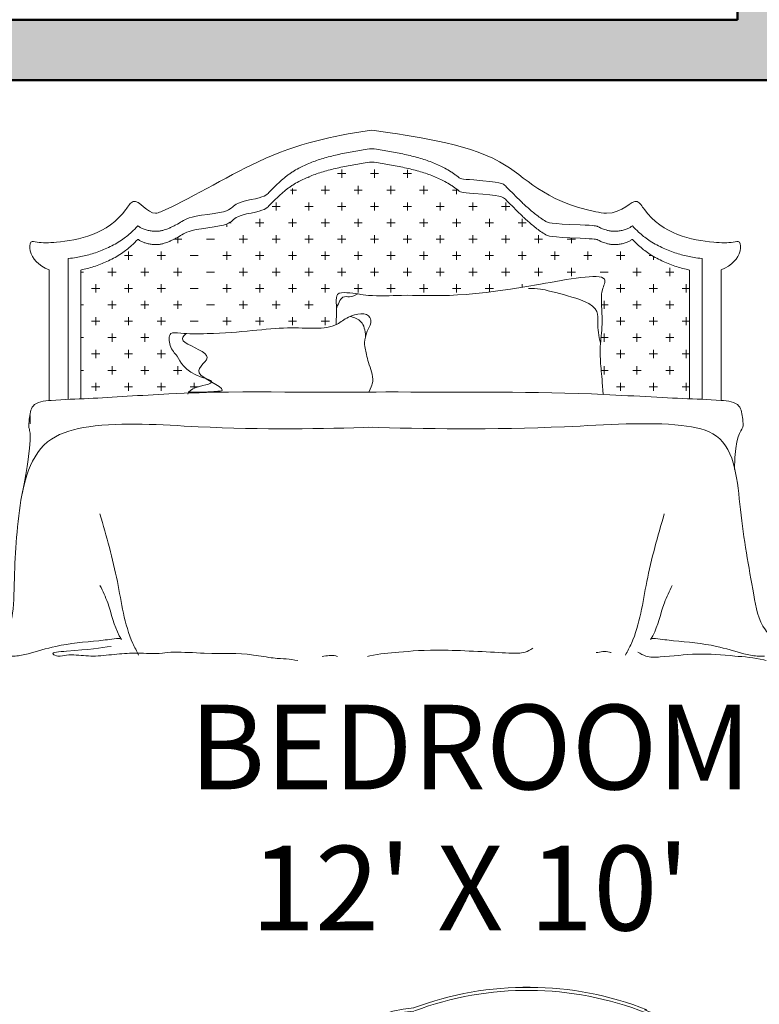
# Model space of a CAD drawing. Units: inches. Extents: x 1771 to 3025, y 319 to 889.
# Tile 10 of 35: x 1978 to 2040, y 713 to 795. Entities that reach past the tile are written whole.
import ezdxf

# ---------------------------------------------------------------- set-up
doc = ezdxf.new("R2010")
doc.units = ezdxf.units.IN
doc.header["$MEASUREMENT"] = 0
doc.set_wipeout_variables(frame=1)
for name, color, linetype, lineweight in [('A-AREA-IDEN', 241, 'Continuous', 25), ('A-FURN', 8, 'Continuous', 18), ('A-WALL', 7, 'Continuous', 50), ('A-WALL-PATT', 254, 'Continuous', 13)]:
    doc.layers.add(name, color=color, linetype=linetype, lineweight=lineweight)
doc.styles.get("Standard").update_dxf_attribs({"font": 'arial.ttf'})

# ---------------------------------------------------------------- blocks, each defined once
blk = doc.blocks.new('A$C3F6F0378')
for p, q in [((1262.2, 944.7), (1262.2, 960.5)), ((1325.7, 944.7), (1325.7, 960.5)), ((1389.2, 944.7), (1389.2, 959.9)), ((1198.7, 944.7), (1198.7, 946.2)), ((1254.2, 952.6), (1270.1, 952.6)), ((1317.7, 952.6), (1333.6, 952.6)), ((1381.2, 952.6), (1397.1, 952.6)), ((1162.7, 920.9), (1174.9, 920.9)), ((1166.9, 912.9), (1166.9, 924)), ((1222.5, 920.9), (1238.4, 920.9)), ((1230.4, 912.9), (1230.4, 928.8)), ((1286, 920.9), (1301.9, 920.9)), ((1293.9, 912.9), (1293.9, 928.8)), ((1349.5, 920.9), (1365.4, 920.9)), ((1357.4, 912.9), (1357.4, 928.8)), ((1413, 920.9), (1428.9, 920.9)), ((1420.9, 912.9), (1420.9, 928.8)), ((1476.5, 920.9), (1485.8, 920.9)), ((1484.4, 912.9), (1484.4, 921.6)), ((1135.2, 881.2), (1135.2, 897)), ((1198.7, 881.2), (1198.7, 897)), ((1262.2, 881.2), (1262.2, 897)), ((1325.7, 881.2), (1325.7, 897)), ((1389.2, 881.2), (1389.2, 897)), ((1452.7, 881.2), (1452.7, 897)), ((1516.2, 881.2), (1516.2, 897)), ((1579.7, 881.2), (1579.7, 897)), ((1127.2, 889.1), (1143.1, 889.1)), ((1190.7, 889.1), (1206.6, 889.1)), ((1254.2, 889.1), (1270.1, 889.1)), ((1317.7, 889.1), (1333.6, 889.1)), ((1381.2, 889.1), (1397.1, 889.1)), ((1444.7, 889.1), (1460.6, 889.1)), ((1508.2, 889.1), (1524.1, 889.1)), ((1571.7, 889.1), (1587.6, 889.1)), ((1103.4, 849.4), (1103.4, 865.3)), ((1166.9, 849.4), (1166.9, 865.3)), ((1230.4, 849.4), (1230.4, 865.3)), ((1293.9, 849.4), (1293.9, 865.3)), ((1357.4, 849.4), (1357.4, 865.3)), ((1420.9, 849.4), (1420.9, 865.3)), ((1484.4, 849.4), (1484.4, 865.3)), ((1547.9, 849.4), (1547.9, 865.3)), ((1611.4, 849.4), (1611.4, 865.3)), ((1039.9, 849.4), (1039.9, 855.2)), ((1044.6, 857.4), (1047.9, 857.4)), ((1095.5, 857.4), (1111.4, 857.4)), ((1159, 857.4), (1174.9, 857.4)), ((1222.5, 857.4), (1238.4, 857.4)), ((1286, 857.4), (1301.9, 857.4)), ((1349.5, 857.4), (1365.4, 857.4)), ((1413, 857.4), (1428.9, 857.4)), ((1476.5, 857.4), (1492.4, 857.4)), ((1540, 857.4), (1555.9, 857.4)), ((1603.5, 857.4), (1619.4, 857.4)), ((937.5, 825.6), (952.6, 825.6)), ((944.7, 817.7), (944.7, 829.4)), ((1000.2, 825.6), (1016.1, 825.6)), ((1063.7, 825.6), (1079.6, 825.6)), ((1071.7, 817.7), (1071.7, 833.5)), ((1127.2, 825.6), (1143.1, 825.6)), ((1135.2, 817.7), (1135.2, 833.5)), ((1190.7, 825.6), (1206.6, 825.6)), ((1198.7, 817.7), (1198.7, 833.5)), ((1254.2, 825.6), (1270.1, 825.6)), ((1262.2, 817.7), (1262.2, 833.5)), ((1317.7, 825.6), (1333.6, 825.6)), ((1325.7, 817.7), (1325.7, 833.5)), ((1381.2, 825.6), (1397.1, 825.6)), ((1389.2, 817.7), (1389.2, 833.5)), ((1444.7, 825.6), (1460.6, 825.6)), ((1452.7, 817.7), (1452.7, 833.5)), ((1508.2, 825.6), (1524.1, 825.6)), ((1516.2, 817.7), (1516.2, 833.5)), ((1571.7, 825.6), (1587.6, 825.6)), ((1579.7, 817.7), (1579.7, 833.5)), ((1635.2, 825.6), (1651.1, 825.6)), ((1643.2, 817.7), (1643.2, 833.5)), ((1698.7, 825.6), (1714.6, 825.6)), ((1706.7, 817.7), (1706.7, 828.2)), ((849.4, 785.9), (849.4, 801.8)), ((881.2, 817.7), (881.2, 818.8)), ((912.9, 785.9), (912.9, 801.8)), ((1039.9, 785.9), (1039.9, 801.8)), ((1103.4, 785.9), (1103.4, 801.8)), ((1166.9, 785.9), (1166.9, 801.8)), ((1230.4, 785.9), (1230.4, 801.8)), ((1293.9, 785.9), (1293.9, 801.8)), ((1357.4, 785.9), (1357.4, 801.8)), ((1420.9, 785.9), (1420.9, 801.8)), ((1484.4, 785.9), (1484.4, 801.8)), ((1547.9, 785.9), (1547.9, 801.8)), ((1611.4, 785.9), (1611.4, 801.8)), ((1674.9, 785.9), (1674.9, 801.8)), ((1738.4, 785.9), (1738.4, 801.8)), ((1770.2, 818.9), (1770.2, 818.9)), ((1801.9, 785.9), (1801.9, 801.8)), ((841.5, 793.9), (857.4, 793.9)), ((905, 793.9), (920.9, 793.9)), ((968.5, 793.9), (984.4, 793.9)), ((1032, 793.9), (1047.9, 793.9)), ((1095.5, 793.9), (1111.4, 793.9)), ((1159, 793.9), (1174.9, 793.9)), ((1222.5, 793.9), (1238.4, 793.9)), ((1286, 793.9), (1301.9, 793.9)), ((1349.5, 793.9), (1365.4, 793.9)), ((1413, 793.9), (1428.9, 793.9)), ((1476.5, 793.9), (1492.4, 793.9)), ((1540, 793.9), (1555.9, 793.9)), ((1603.5, 793.9), (1619.4, 793.9)), ((1667, 793.9), (1682.9, 793.9)), ((1730.5, 793.9), (1746.4, 793.9)), ((1794, 793.9), (1809.9, 793.9)), ((1857.5, 793.9), (1863, 793.9)), ((1865.4, 785.9), (1865.4, 792.4)), ((817.7, 754.2), (817.7, 770)), ((881.2, 754.2), (881.2, 770)), ((944.7, 754.2), (944.7, 770)), ((1071.7, 754.2), (1071.7, 770)), ((1135.2, 754.2), (1135.2, 770)), ((1198.7, 754.2), (1198.7, 770)), ((1262.2, 754.2), (1262.2, 770)), ((1325.7, 754.2), (1325.7, 770)), ((1389.2, 754.2), (1389.2, 770)), ((1452.7, 754.2), (1452.7, 770)), ((1516.2, 754.2), (1516.2, 770)), ((1579.7, 754.2), (1579.7, 770)), ((1643.2, 754.2), (1643.2, 770)), ((1706.7, 754.2), (1706.7, 770)), ((1833.7, 754.2), (1833.7, 770)), ((1897.2, 754.2), (1897.2, 770)), ((757.1, 762.1), (762.1, 762.1)), ((809.7, 762.1), (825.6, 762.1)), ((873.2, 762.1), (889.1, 762.1)), ((936.7, 762.1), (952.6, 762.1)), ((1000.2, 762.1), (1016.1, 762.1)), ((1063.7, 762.1), (1079.6, 762.1)), ((1127.2, 762.1), (1143.1, 762.1)), ((1190.7, 762.1), (1206.6, 762.1)), ((1254.2, 762.1), (1270.1, 762.1)), ((1317.7, 762.1), (1333.6, 762.1)), ((1381.2, 762.1), (1397.1, 762.1)), ((1444.7, 762.1), (1460.6, 762.1)), ((1508.2, 762.1), (1524.1, 762.1)), ((1571.7, 762.1), (1587.6, 762.1)), ((1635.2, 762.1), (1651.1, 762.1)), ((1698.7, 762.1), (1714.6, 762.1)), ((1762.2, 762.1), (1778.1, 762.1)), ((1825.7, 762.1), (1841.6, 762.1)), ((1889.2, 762.1), (1905.1, 762.1)), ((778, 730.4), (793.9, 730.4)), ((785.9, 722.4), (785.9, 738.3)), ((841.5, 730.4), (857.4, 730.4)), ((849.4, 722.4), (849.4, 738.3)), ((905, 730.4), (920.9, 730.4)), ((912.9, 722.4), (912.9, 738.3)), ((968.5, 730.4), (984.4, 730.4)), ((1032, 730.4), (1047.9, 730.4)), ((1039.9, 722.4), (1039.9, 738.3)), ((1095.5, 730.4), (1111.4, 730.4)), ((1103.4, 722.4), (1103.4, 738.3)), ((1159, 730.4), (1174.9, 730.4)), ((1166.9, 722.4), (1166.9, 738.3)), ((1222.5, 730.4), (1238.4, 730.4)), ((1230.4, 722.4), (1230.4, 738.3)), ((1286, 730.4), (1301.9, 730.4)), ((1293.9, 722.4), (1293.9, 738.3)), ((1349.5, 730.4), (1365.4, 730.4)), ((1357.4, 722.4), (1357.4, 738.3)), ((1413, 730.4), (1428.9, 730.4)), ((1420.9, 722.4), (1420.9, 738.3)), ((1476.5, 730.4), (1492.4, 730.4)), ((1484.4, 722.4), (1484.4, 738.3)), ((1540, 730.4), (1555.9, 730.4)), ((1547.9, 723.4), (1547.9, 738.3)), ((1611.4, 732.6), (1611.4, 738.3)), ((1794, 730.4), (1809.9, 730.4)), ((1801.9, 722.4), (1801.9, 738.3)), ((1857.5, 730.4), (1873.4, 730.4)), ((1865.4, 722.4), (1865.4, 738.3)), ((1921, 730.4), (1935.3, 730.4)), ((1928.9, 722.4), (1928.9, 738.3)), ((817.7, 690.7), (817.7, 706.5)), ((881.2, 690.7), (881.2, 706.5)), ((944.7, 690.7), (944.7, 706.5)), ((1071.7, 690.7), (1071.7, 706.5)), ((1135.2, 690.7), (1135.2, 706.5)), ((1198.7, 690.7), (1198.7, 706.5)), ((1770.2, 690.7), (1770.2, 706.5)), ((1833.7, 690.7), (1833.7, 706.5)), ((1897.2, 690.7), (1897.2, 706.5)), ((757.1, 698.6), (762.1, 698.6)), ((809.7, 698.6), (825.6, 698.6)), ((873.2, 698.6), (889.1, 698.6)), ((936.7, 698.6), (952.6, 698.6)), ((1000.2, 698.6), (1016.1, 698.6)), ((1063.7, 698.6), (1079.6, 698.6)), ((1127.2, 698.6), (1143.1, 698.6)), ((1190.7, 698.6), (1206.6, 698.6)), ((1765.2, 698.6), (1778.1, 698.6)), ((1825.7, 698.6), (1841.6, 698.6)), ((1889.2, 698.6), (1905.1, 698.6)), ((785.9, 658.9), (785.9, 674.8)), ((849.4, 658.9), (849.4, 674.8)), ((912.9, 658.9), (912.9, 674.8)), ((1039.9, 658.9), (1039.9, 674.8)), ((1103.4, 658.9), (1103.4, 674.8)), ((1166.9, 658.9), (1166.9, 674.8)), ((1230.4, 658.9), (1230.4, 674.8)), ((1801.9, 658.9), (1801.9, 674.8)), ((1865.4, 658.9), (1865.4, 674.8)), ((1928.9, 658.9), (1928.9, 674.8)), ((778, 666.9), (793.9, 666.9)), ((841.5, 666.9), (857.4, 666.9)), ((905, 666.9), (920.9, 666.9)), ((968.5, 666.9), (984.4, 666.9)), ((1032, 666.9), (1047.9, 666.9)), ((1095.5, 666.9), (1111.4, 666.9)), ((1159, 666.9), (1174.9, 666.9)), ((1222.5, 666.9), (1238.4, 666.9)), ((1794, 666.9), (1809.9, 666.9)), ((1857.5, 666.9), (1873.4, 666.9)), ((1921, 666.9), (1935.3, 666.9)), ((757.1, 635.1), (762.1, 635.1)), ((809.7, 635.1), (825.6, 635.1)), ((817.7, 627.2), (817.7, 643)), ((873.2, 635.1), (889.1, 635.1)), ((881.2, 627.2), (881.2, 643)), ((1764.2, 635.1), (1778.1, 635.1)), ((1770.2, 627.2), (1770.2, 643)), ((1825.7, 635.1), (1841.6, 635.1)), ((1833.7, 627.2), (1833.7, 643)), ((1889.2, 635.1), (1905.1, 635.1)), ((1897.2, 627.2), (1897.2, 643)), ((785.9, 595.4), (785.9, 611.3)), ((849.4, 595.4), (849.4, 611.3)), ((912.9, 595.4), (912.9, 611.3)), ((1801.9, 595.4), (1801.9, 611.3)), ((1865.4, 595.4), (1865.4, 611.3)), ((1928.9, 595.4), (1928.9, 611.3)), ((778, 603.4), (793.9, 603.4)), ((841.5, 603.4), (857.4, 603.4)), ((905, 603.4), (920.9, 603.4)), ((1794, 603.4), (1809.9, 603.4)), ((1857.5, 603.4), (1873.4, 603.4)), ((1921, 603.4), (1935.3, 603.4)), ((817.7, 563.7), (817.7, 579.5)), ((881.2, 563.7), (881.2, 579.5)), ((944.7, 563.7), (944.7, 579.5)), ((1770.2, 563.7), (1770.2, 579.5)), ((1833.7, 563.7), (1833.7, 579.5)), ((1897.2, 563.7), (1897.2, 579.5)), ((757.1, 571.6), (762.1, 571.6)), ((809.7, 571.6), (825.6, 571.6)), ((873.2, 571.6), (889.1, 571.6)), ((936.7, 571.6), (952.6, 571.6)), ((1764.5, 571.6), (1778.1, 571.6)), ((1825.7, 571.6), (1841.6, 571.6)), ((1889.2, 571.6), (1905.1, 571.6)), ((778, 539.9), (793.9, 539.9)), ((785.9, 531.9), (785.9, 547.8)), ((841.5, 539.9), (857.4, 539.9)), ((849.4, 531.9), (849.4, 547.8)), ((905, 539.9), (920.9, 539.9)), ((912.9, 531.9), (912.9, 547.8)), ((968.5, 539.9), (984.4, 539.9)), ((976.4, 536.8), (976.4, 547.8)), ((1794, 539.9), (1809.9, 539.9)), ((1801.9, 531.9), (1801.9, 547.8)), ((1857.5, 539.9), (1873.4, 539.9)), ((1865.4, 531.9), (1865.4, 547.8)), ((1921, 539.9), (1935.3, 539.9)), ((1928.9, 531.9), (1928.9, 547.8)), ((658.9, 468.4), (658.9, 484.3))]:
    blk.add_line(p, q)
at = {"ltscale": 20}
for p, q in [((732.5, 788.3), (732.5, 515.5)), ((1959.8, 788.3), (1959.8, 515.7)), ((695.7, 766.2), (695.7, 513.2)), ((757.1, 766), (757.1, 516.6)), ((1935.3, 766), (1935.3, 516.7)), ((1996.6, 766.2), (1996.6, 513.5))]:
    blk.add_line(p, q, dxfattribs=at)
for centre in [(1320.3, 981.3), (1320.4, 945.7), (1320.4, 919.9)]:
    blk.add_arc(centre, 55.2, 80.5605, 99.4395, dxfattribs=at)
for points, knots in [([(695.7, 766.2), (675.2, 775.8), (657.2, 791.6), (658.6, 824.3), (675.7, 817.9), (731.9, 819.9), (817.7, 836.7), (863.4, 913.8), (889.3, 869.9), (957.4, 896.6), (1128.9, 1003.6), (1245.7, 1025), (1311.4, 1035.8)], [12.417853, 12.417853, 12.417853, 12.417853, 68.394536, 90.665986, 114.156853, 157.554067, 281.869614, 298.858744, 338.737111, 347.060176, 470.423438, 625.498764, 625.498764, 625.498764, 625.498764]), ([(1996.6, 766.2), (2017.1, 775.8), (2035.1, 791.6), (2033.8, 824.3), (2016.6, 817.9), (1960.4, 819.9), (1874.7, 836.7), (1829, 913.8), (1803, 869.9), (1652.5, 896.6), (1584, 1003.6), (1395.1, 1025), (1329.4, 1035.8)], [12.417853, 12.417853, 12.417853, 12.417853, 68.394536, 90.665986, 114.156853, 157.554067, 281.869614, 298.858744, 338.737111, 347.060176, 470.423438, 625.498764, 625.498764, 625.498764, 625.498764]), ([(867.4, 851.3), (868.1, 850.9), (868.9, 850.4), (871.2, 849.1), (872.9, 848.2), (876.8, 846.3), (879, 845.4), (884, 843.6), (886.7, 842.8), (892, 841.7), (894.6, 841.4), (898.4, 841.1), (899.4, 841), (901.2, 841), (901.9, 841), (903.1, 841), (903.7, 841.1), (904.8, 841.1), (905.4, 841.2), (907, 841.3), (908.1, 841.4), (911.6, 841.9), (913.8, 842.3), (917.8, 843.3), (919.6, 843.9), (922.7, 844.9), (924.1, 845.5), (926.6, 846.4), (927.6, 846.9), (928.8, 847.4), (929.1, 847.5), (929.7, 847.8), (929.9, 847.9), (930.7, 848.2), (931.3, 848.5), (932.9, 849.2), (933.9, 849.7), (937.1, 851.3), (939.2, 852.3), (945.3, 855.5), (949.2, 857.8), (959.8, 864.4), (966.2, 869), (1040, 878.3), (1045.6, 883.1), (1056.3, 892.7), (1061.3, 897.5), (1112.2, 907), (1116.8, 911.6), (1125.6, 920.6), (1129.9, 924.9), (1138.3, 933), (1142.3, 936.8), (1148.2, 942), (1150, 943.5), (1153.3, 946.3), (1154.7, 947.4), (1157, 949.2), (1157.9, 949.9), (1159.7, 951.2), (1160.6, 951.8), (1163.4, 953.8), (1165.3, 955), (1171, 958.7), (1174.9, 961), (1186, 967), (1193.5, 970.4), (1209.3, 976.7), (1217.6, 979.5), (1235, 984.7), (1244, 987), (1262.7, 991.3), (1272.4, 993.3), (1291.8, 996.9), (1301.5, 998.6), (1311.3, 1000.2)], [328.6705, 328.6705, 328.6705, 328.6705, 329.609368, 329.609368, 331.487103, 331.487103, 333.620342, 333.620342, 335.753581, 335.753581, 337.507866, 337.507866, 338.182373, 338.182373, 338.607397, 338.607397, 338.959312, 338.959312, 339.311227, 339.311227, 340.015058, 340.015058, 341.722742, 341.722742, 343.430427, 343.430427, 345.138111, 345.138111, 346.845796, 346.845796, 347.37881, 347.37881, 347.911824, 347.911824, 348.977853, 348.977853, 351.109909, 351.109909, 355.374023, 355.374023, 363.902249, 363.902249, 379.258481, 379.258481, 394.614712, 394.614712, 409.970944, 409.970944, 425.327175, 425.327175, 440.683406, 440.683406, 456.039638, 456.039638, 463.285514, 463.285514, 469.01116, 469.01116, 472.593, 472.593, 476.17484, 476.17484, 483.338521, 483.338521, 497.665882, 497.665882, 522.309302, 522.309302, 546.952723, 546.952723, 571.596143, 571.596143, 596.239564, 596.239564, 619.876409, 619.876409, 619.876409, 619.876409]), ([(1824.9, 851.3), (1824.2, 850.9), (1823.5, 850.4), (1821.1, 849.1), (1819.5, 848.2), (1815.6, 846.3), (1813.3, 845.4), (1808.4, 843.6), (1805.7, 842.8), (1800.3, 841.7), (1797.7, 841.4), (1794, 841.1), (1792.9, 841), (1791.2, 841), (1790.5, 841), (1789.2, 841), (1788.6, 841.1), (1787.5, 841.1), (1787, 841.2), (1785.3, 841.3), (1784.3, 841.4), (1780.8, 841.9), (1778.6, 842.3), (1774.6, 843.3), (1772.8, 843.9), (1769.6, 844.9), (1768.2, 845.5), (1765.8, 846.4), (1764.7, 846.9), (1763.5, 847.4), (1763.2, 847.5), (1762.7, 847.8), (1762.4, 847.9), (1761.6, 848.2), (1761.1, 848.5), (1759.5, 849.2), (1758.4, 849.7), (1755.2, 851.3), (1753.2, 852.3), (1664.6, 855.5), (1660.7, 857.8), (1650.1, 864.4), (1643.7, 869), (1631.7, 878.3), (1626.1, 883.1), (1615.5, 892.7), (1610.4, 897.5), (1600.8, 907), (1596.2, 911.6), (1587.3, 920.6), (1583, 924.9), (1574.7, 933), (1570.6, 936.8), (1492.6, 942), (1490.8, 943.5), (1487.5, 946.3), (1486.1, 947.4), (1483.8, 949.2), (1482.9, 949.9), (1481.1, 951.2), (1480.2, 951.8), (1477.4, 953.8), (1475.5, 955), (1469.8, 958.7), (1465.9, 961), (1454.8, 967), (1447.3, 970.4), (1431.5, 976.7), (1423.2, 979.5), (1405.8, 984.7), (1396.8, 987), (1378.1, 991.3), (1368.4, 993.3), (1349, 996.9), (1339.3, 998.6), (1329.5, 1000.2)], [328.6705, 328.6705, 328.6705, 328.6705, 329.609368, 329.609368, 331.487103, 331.487103, 333.620342, 333.620342, 335.753581, 335.753581, 337.507866, 337.507866, 338.182373, 338.182373, 338.607397, 338.607397, 338.959312, 338.959312, 339.311227, 339.311227, 340.015058, 340.015058, 341.722742, 341.722742, 343.430427, 343.430427, 345.138111, 345.138111, 346.845796, 346.845796, 347.37881, 347.37881, 347.911824, 347.911824, 348.977853, 348.977853, 351.109909, 351.109909, 355.374023, 355.374023, 363.902249, 363.902249, 379.258481, 379.258481, 394.614712, 394.614712, 409.970943, 409.970943, 425.327175, 425.327175, 440.683406, 440.683406, 456.039637, 456.039637, 463.285514, 463.285514, 469.011154, 469.011154, 472.592992, 472.592992, 476.17483, 476.17483, 483.338506, 483.338506, 497.665857, 497.665857, 522.309275, 522.309275, 546.952693, 546.952693, 571.59611, 571.59611, 596.239528, 596.239528, 619.876409, 619.876409, 619.876409, 619.876409]), ([(867.4, 825.4), (868.1, 825), (868.9, 824.6), (871.2, 823.2), (872.9, 822.3), (876.8, 820.5), (879, 819.5), (884, 817.8), (886.7, 817), (892, 815.9), (894.6, 815.5), (898.4, 815.2), (899.4, 815.2), (901.2, 815.2), (901.9, 815.2), (903.1, 815.2), (903.7, 815.2), (904.8, 815.3), (905.4, 815.3), (907, 815.4), (908.1, 815.5), (911.6, 816), (913.8, 816.5), (917.8, 817.5), (919.6, 818), (922.7, 819.1), (924.1, 819.6), (926.6, 820.6), (927.6, 821), (928.8, 821.5), (929.1, 821.7), (929.7, 821.9), (929.9, 822), (930.7, 822.4), (931.3, 822.6), (932.9, 823.4), (933.9, 823.9), (937.1, 825.4), (939.2, 826.4), (945.3, 829.7), (949.2, 832), (959.8, 838.6), (966.2, 843.1), (1040, 852.4), (1045.6, 857.2), (1056.3, 866.8), (1061.3, 871.6), (1112.2, 881.1), (1116.8, 885.7), (1125.6, 894.7), (1129.9, 899), (1138.3, 907.1), (1142.3, 910.9), (1148.2, 916.1), (1150, 917.7), (1153.3, 920.4), (1154.7, 921.5), (1157, 923.3), (1157.9, 924), (1159.7, 925.3), (1160.6, 926), (1163.4, 927.9), (1165.3, 929.2), (1171, 932.8), (1174.9, 935.2), (1186, 941.1), (1193.5, 944.6), (1209.3, 950.8), (1217.6, 953.7), (1235, 958.8), (1244, 961.2), (1262.7, 965.5), (1272.4, 967.4), (1291.8, 971), (1301.5, 972.7), (1311.3, 974.3)], [328.6705, 328.6705, 328.6705, 328.6705, 329.609368, 329.609368, 331.487103, 331.487103, 333.620342, 333.620342, 335.753581, 335.753581, 337.507866, 337.507866, 338.182373, 338.182373, 338.607397, 338.607397, 338.959312, 338.959312, 339.311227, 339.311227, 340.015058, 340.015058, 341.722742, 341.722742, 343.430427, 343.430427, 345.138111, 345.138111, 346.845796, 346.845796, 347.37881, 347.37881, 347.911824, 347.911824, 348.977853, 348.977853, 351.109909, 351.109909, 355.374023, 355.374023, 363.902249, 363.902249, 379.258481, 379.258481, 394.614712, 394.614712, 409.970944, 409.970944, 425.327175, 425.327175, 440.683406, 440.683406, 456.039638, 456.039638, 463.285514, 463.285514, 469.01116, 469.01116, 472.593, 472.593, 476.17484, 476.17484, 483.338521, 483.338521, 497.665882, 497.665882, 522.309302, 522.309302, 546.952723, 546.952723, 571.596143, 571.596143, 596.239564, 596.239564, 619.876409, 619.876409, 619.876409, 619.876409]), ([(1824.9, 825.4), (1824.2, 825), (1823.5, 824.6), (1821.1, 823.2), (1819.5, 822.3), (1815.6, 820.5), (1813.3, 819.5), (1808.4, 817.8), (1805.7, 817), (1800.3, 815.9), (1797.7, 815.5), (1794, 815.2), (1792.9, 815.2), (1791.2, 815.2), (1790.5, 815.2), (1789.2, 815.2), (1788.6, 815.2), (1787.5, 815.3), (1787, 815.3), (1785.3, 815.4), (1784.3, 815.5), (1780.8, 816), (1778.6, 816.5), (1774.6, 817.5), (1772.8, 818), (1769.6, 819.1), (1768.2, 819.6), (1765.8, 820.6), (1764.7, 821), (1763.5, 821.5), (1763.2, 821.7), (1762.7, 821.9), (1762.4, 822), (1761.6, 822.4), (1761.1, 822.6), (1759.5, 823.4), (1758.4, 823.9), (1755.2, 825.4), (1753.2, 826.4), (1664.6, 829.7), (1660.7, 832), (1650.1, 838.6), (1643.7, 843.1), (1631.7, 852.4), (1626.1, 857.2), (1615.5, 866.8), (1610.4, 871.6), (1600.8, 881.1), (1596.2, 885.7), (1587.3, 894.7), (1583, 899), (1574.7, 907.1), (1570.6, 910.9), (1492.6, 916.1), (1490.8, 917.7), (1487.5, 920.4), (1486.1, 921.5), (1483.8, 923.3), (1482.9, 924), (1481.1, 925.3), (1480.2, 926), (1477.4, 927.9), (1475.5, 929.2), (1469.8, 932.8), (1465.9, 935.2), (1454.8, 941.1), (1447.3, 944.6), (1431.5, 950.8), (1423.2, 953.7), (1405.8, 958.8), (1396.8, 961.2), (1378.1, 965.5), (1368.4, 967.4), (1349, 971), (1339.3, 972.7), (1329.5, 974.3)], [328.6705, 328.6705, 328.6705, 328.6705, 329.609368, 329.609368, 331.487103, 331.487103, 333.620342, 333.620342, 335.753581, 335.753581, 337.507866, 337.507866, 338.182373, 338.182373, 338.607397, 338.607397, 338.959312, 338.959312, 339.311227, 339.311227, 340.015058, 340.015058, 341.722742, 341.722742, 343.430427, 343.430427, 345.138111, 345.138111, 346.845796, 346.845796, 347.37881, 347.37881, 347.911824, 347.911824, 348.977853, 348.977853, 351.109909, 351.109909, 355.374023, 355.374023, 363.902249, 363.902249, 379.258481, 379.258481, 394.614712, 394.614712, 409.970943, 409.970943, 425.327175, 425.327175, 440.683406, 440.683406, 456.039637, 456.039637, 463.285514, 463.285514, 469.011154, 469.011154, 472.592992, 472.592992, 476.17483, 476.17483, 483.338506, 483.338506, 497.665857, 497.665857, 522.309275, 522.309275, 546.952693, 546.952693, 571.59611, 571.59611, 596.239528, 596.239528, 619.876409, 619.876409, 619.876409, 619.876409]), ([(732.5, 788.3), (744.7, 789.4), (752.5, 790.8), (768.6, 794.5), (777, 796.7), (793.9, 802.3), (802.4, 805.7), (819.3, 813.7), (827.7, 818.4), (842.6, 828.5), (849.2, 833.6), (859.6, 843.1), (863.6, 847.1), (867.4, 851.3)], [179.330708, 179.330708, 179.330708, 179.330708, 196.086144, 196.086144, 213.445516, 213.445516, 230.804888, 230.804888, 248.16426, 248.16426, 262.451931, 262.451931, 271.832526, 271.832526, 271.832526, 271.832526]), ([(1959.8, 788.3), (1947.6, 789.5), (1939.9, 790.9), (1923.7, 794.5), (1915.4, 796.7), (1898.5, 802.3), (1889.9, 805.7), (1873, 813.7), (1864.6, 818.4), (1849.7, 828.5), (1843.2, 833.6), (1832.8, 843.1), (1828.8, 847.1), (1824.9, 851.3)], [179.400376, 179.400376, 179.400376, 179.400376, 196.086144, 196.086144, 213.445516, 213.445516, 230.804888, 230.804888, 248.16426, 248.16426, 262.451931, 262.451931, 271.832526, 271.832526, 271.832526, 271.832526]), ([(757.1, 766), (758.2, 766.3), (759.3, 766.5), (768.6, 768.6), (777, 770.9), (793.9, 776.5), (802.4, 779.8), (819.3, 787.9), (827.7, 792.6), (842.6, 802.7), (849.2, 807.8), (859.6, 817.2), (863.6, 821.2), (867.4, 825.4)], [193.740688, 193.740688, 193.740688, 193.740688, 196.086144, 196.086144, 213.445516, 213.445516, 230.804888, 230.804888, 248.16426, 248.16426, 262.451931, 262.451931, 271.832526, 271.832526, 271.832526, 271.832526]), ([(1935.3, 766), (1934.2, 766.3), (1933.1, 766.5), (1923.7, 768.6), (1915.4, 770.9), (1898.5, 776.5), (1889.9, 779.8), (1873, 787.9), (1864.6, 792.6), (1849.7, 802.7), (1843.2, 807.8), (1832.8, 817.2), (1828.8, 821.2), (1824.9, 825.4)], [193.740688, 193.740688, 193.740688, 193.740688, 196.086144, 196.086144, 213.445516, 213.445516, 230.804888, 230.804888, 248.16426, 248.16426, 262.451931, 262.451931, 271.832526, 271.832526, 271.832526, 271.832526])]:
    blk.add_open_spline(points, degree=3, knots=knots, dxfattribs=at)
at = {"ltscale": 5}
for points, knots in [([(1251.5, 660.5), (1251.8, 673.8), (1252.2, 692.2), (1250.9, 722.8), (1282.7, 722.3), (1319.1, 713.9), (1424.2, 721.3), (1489.1, 705.6), (1786.5, 765.5), (1764.9, 728.8), (1764.7, 698.2), (1767.9, 658.9), (1761, 614.3), (1764.1, 574.4), (1766.6, 548.7), (1767.9, 525.2)], [3.603347, 3.603347, 3.603347, 3.603347, 60.838375, 82.182907, 107.012175, 163.177093, 249.239778, 501.114283, 577.787612, 607.274607, 630.949286, 706.159707, 762.92633, 812.910096, 867.096105, 867.096105, 867.096105, 867.096105]), ([(1623.4, 730.2), (1631.2, 730.2), (1644.4, 730.3), (1665.2, 725.1), (1763.6, 700.2), (1754.4, 664.8), (1760.1, 637.6), (1763, 624), (1763.1, 623.6)], [0, 0, 0, 0, 31.268494, 53.71641, 83.24833, 138.583941, 192.96698, 194.695488, 194.695488, 194.695488, 194.695488]), ([(1293.1, 719.7), (1288.2, 716.8), (1279.1, 713), (1263.5, 715.9), (1256.5, 703.2), (1253.3, 695), (1251.9, 690.7)], [16.588235, 16.588235, 16.588235, 16.588235, 39.368234, 56.465167, 72.647278, 91.317886, 91.317886, 91.317886, 91.317886]), ([(964.3, 525.7), (965, 536.9), (1030.6, 547.7), (956.6, 565.4), (948, 599.2), (929.2, 612.7), (925.7, 647.1), (951.8, 642.5), (1054.9, 642.1), (1162.4, 661.2), (1239, 646.9), (1276.3, 678.9), (1316.3, 686.5), (1319.5, 660.6), (1309.9, 647.1), (1305, 623.9), (1309.2, 608.7), (1312.5, 586.6), (1326.7, 553.1), (1318.1, 538.8), (1314.8, 529.7)], [33.020195, 33.020195, 33.020195, 33.020195, 57.294753, 90.473933, 194.149416, 257.058105, 304.592565, 338.383824, 389.043604, 577.649845, 759.359611, 813.032269, 898.973184, 920.659088, 956.429806, 1000.911745, 1042.797508, 1121.842246, 1191.460876, 1213.109701, 1213.109701, 1213.109701, 1213.109701]), ([(1278.5, 676.1), (1286.8, 673.9), (1304.1, 667.4), (1307.6, 649.1), (1308.3, 637.8)], [13.535772, 13.535772, 13.535772, 13.535772, 45.871957, 87.312392, 87.312392, 87.312392, 87.312392]), ([(961.3, 642.9), (955.5, 638.3), (944, 626.2), (1030.7, 599.4), (953, 567.4), (1038.4, 539.7), (1029.3, 530.5), (966, 529.3)], [5.952535, 5.952535, 5.952535, 5.952535, 29.258845, 70.114919, 115.518645, 162.322231, 169.813565, 169.813565, 169.813565, 169.813565]), ([(643.4, 331.9), (665.9, 445.8), (654.5, 454.3), (658, 480.9), (661.2, 509.9), (714.1, 515.4), (786.5, 516.7), (1040.5, 536.6), (1224.6, 526.5), (1352.9, 530.4)], [0, 0, 0, 0, 32.681627, 48.455722, 75.25348, 112.004017, 183.381957, 310.642358, 688.088714, 688.088714, 688.088714, 688.088714]), ([(2022.3, 380), (2023.2, 448.3), (2041.3, 454.3), (2037.8, 480.9), (2034.7, 509.9), (1981.7, 515.4), (1909.3, 516.7), (1667.8, 533.2), (1476.1, 527.9), (1347.4, 530.2)], [0, 0, 0, 0, 32.681627, 48.455722, 75.25348, 112.004017, 183.381957, 310.642358, 588.939547, 588.939547, 588.939547, 588.939547]), ([(594.1, 49), (601.1, 55.3), (626, 78.1), (628.7, 172), (631.8, 287.1), (663.1, 436.6), (808.3, 475), (1037.5, 455.3), (1227.9, 458.5), (1322.1, 461.7)], [0, 0, 0, 0, 28.320233, 100.953775, 269.820348, 420.691469, 489.161544, 656.134073, 940.569207, 940.569207, 940.569207, 940.569207]), ([(2101.8, 49), (2094.8, 55.3), (2069.8, 78.1), (2053.9, 172), (2031.7, 287.1), (2023.3, 445.1), (1887.5, 475), (1637.7, 455.3), (1416.4, 458.5), (1314.5, 461.4)], [0, 0, 0, 0, 28.320233, 100.953775, 269.820348, 420.691469, 489.161544, 656.134073, 940.569207, 940.569207, 940.569207, 940.569207]), ([(794.2, 293.6), (806.6, 250.4), (830.4, 167.7), (842.1, 71.7), (865.2, 27.8), (869.1, 20.4)], [0, 0, 0, 0, 135.247847, 258.692787, 283.800228, 283.800228, 283.800228, 283.800228]), ([(1886.4, 293.6), (1874, 250.4), (1850.2, 167.7), (1838.6, 71.7), (1815.4, 27.8), (1811.5, 20.4)], [0, 0, 0, 0, 135.247847, 258.692787, 283.800228, 283.800228, 283.800228, 283.800228]), ([(794.2, 155.1), (799.6, 144.1), (814.7, 112.8), (821.4, 74.6), (834.4, 53), (835.9, 50.7)], [0, 0, 0, 0, 37.234018, 105.386078, 113.844905, 113.844905, 113.844905, 113.844905]), ([(1901.7, 155.1), (1896.3, 144.1), (1881.1, 112.8), (1874.4, 74.6), (1861.4, 53), (1859.9, 50.7)], [0, 0, 0, 0, 37.234018, 105.386078, 113.844905, 113.844905, 113.844905, 113.844905]), ([(615.5, 18.4), (620.3, 18.3), (633.7, 17.9), (664.9, 24.9), (717, 41.9), (776.4, 46.5), (816.6, 50.9), (832.8, 53.1), (835.5, 51), (835.9, 50.7)], [0, 0, 0, 0, 14.447875, 40.468341, 96.220884, 181.018327, 216.046098, 224.609189, 226.185962, 226.185962, 226.185962, 226.185962]), ([(2080.3, 18.4), (2075.6, 18.3), (2062.2, 17.9), (2030.9, 24.9), (1978.8, 41.9), (1919.5, 46.5), (1879.3, 50.9), (1863, 53.1), (1860.4, 51), (1859.9, 50.7)], [0, 0, 0, 0, 14.447875, 40.468341, 96.220884, 181.018327, 216.046098, 224.609189, 226.185962, 226.185962, 226.185962, 226.185962]), ([(815.7, 37.2), (795, 34.1), (767.8, 30.1), (693.6, 25.5), (716, 16.2), (729.8, 21.8), (754.8, 20), (787, 17), (826.3, 22.8), (869.3, 25.1), (905.1, 21.9), (935.5, 27.3), (1029.7, 21.6), (1063.4, 26), (1134.3, 13.3), (1155.4, 13.6), (1169.6, 10.9), (1177, 9.9)], [0, 0, 0, 0, 87.513803, 114.592793, 124.77702, 141.903576, 160.817021, 198.691115, 240.471478, 280.23486, 329.410006, 348.41762, 373.077233, 428.05708, 447.802257, 468.691939, 491.310217, 491.310217, 491.310217, 491.310217]), ([(1224.5, 17.5), (1233.4, 18.9), (1243.5, 21.4), (1252.6, 17.9), (1253.7, 17.5)], [516.212662, 516.212662, 516.212662, 516.212662, 542.681017, 546.007116, 546.007116, 546.007116, 546.007116]), ([(1311.8, 17.5), (1313.3, 17.9), (1334, 23.1), (1377.5, 26.3), (1445.4, 32.7), (1573.8, 24.6), (1614, 23), (1627.1, 30.7), (1632, 33.6)], [590.079786, 590.079786, 590.079786, 590.079786, 594.646549, 651.888327, 725.747367, 797.841373, 826.274406, 843.189267, 843.189267, 843.189267, 843.189267]), ([(1754.5, 25.1), (1763.4, 26.5), (1773.5, 29), (1782.6, 25.5), (1783.6, 25.1)], [516.212662, 516.212662, 516.212662, 516.212662, 542.681017, 546.007116, 546.007116, 546.007116, 546.007116]), ([(2083.5, 9.9), (2082, 10.3), (2061.3, 15.5), (2017.8, 18.7), (1949.9, 25.1), (1893.7, 17), (1853.5, 15.4), (1840.4, 23.1), (1835.5, 26)], [590.079786, 590.079786, 590.079786, 590.079786, 594.646549, 651.888327, 725.747367, 797.841373, 826.274406, 843.189267, 843.189267, 843.189267, 843.189267])]:
    blk.add_open_spline(points, degree=3, knots=knots, dxfattribs=at)
blk = doc.blocks.new('A$C425441F1')
for points in [[(1639.3, 0), (1667.3, 0), (1667.3, 55.3), (1748.6, 55.3), (1748.6, 807.4), (1761.1, 860.7), (1735.7, 880.7), (1703.4, 883.3), (1675.8, 879.6), (1656.2, 873.5), (1635.2, 863.3), (1619.6, 852.6), (1605.1, 839.5), (1596.7, 829.9), (1583.2, 810), (1573.2, 788.1), (1567.6, 767.7), (1566.5, 761.6), (1541.6, 750.9), (1510.7, 736.6), (1488.3, 725.3), (1464.5, 712.2), (1433.4, 693.6), (1409.1, 677.8), (1389.7, 664.2), (1388.2, 683.8), (1383.3, 700), (1376.2, 712), (1365.5, 723.2), (1352, 731.8), (1342.1, 735.4), (1331.7, 738.6), (1325, 742.7), (1317.7, 750.9), (1314.2, 758.8), (1312.9, 767.9), (1315.6, 780.8), (1321.1, 788.9), (1323.4, 793.7), (1323.6, 797.2), (1323.1, 800), (1320.5, 804.5), (1317.8, 806.7), (1317.8, 807.1), (1478.8, 807.1), (1345.8, 1080.7), (1177.3, 1080.7), (1044.3, 807.1), (1211.1, 807.1), (1211.1, 806.7), (1207.8, 803.9), (1205.8, 800.4), (1205.1, 796.3), (1207.6, 788.9), (1211.4, 783.4), (1213.5, 778.7), (1215.3, 769.8), (1215.1, 763.9), (1214.1, 759), (1208.8, 748.5), (1201.9, 741.7), (1195.3, 738), (1185.9, 735.4), (1176, 731.7), (1166.8, 726.4), (1159.9, 720.8), (1156.8, 717.7), (1149.3, 708.1), (1145.7, 701.6), (1143.6, 696.9), (1138.7, 669.7), (1138.7, 651.6), (1140.7, 631.8), (1142.6, 621.6), (1148.5, 600.5), (1162.8, 569), (1176.9, 547.8), (1188.6, 534.2), (1200, 523), (983, 523), (977.7, 522.3), (971.8, 519.6), (965.5, 512.8), (963.3, 506.8), (963, 503), (974.8, 503), (974.8, 3), (1013, 3), (1013, 103), (1053.6, 103), (1052.7, 96.1), (1051.6, 86.5), (1049.3, 63.6), (1048.6, 55.3), (1130.1, 55.3), (1130.1, 0), (1157.9, 0), (1174.1, 55.3), (1623.1, 55.6)], [(778.6, 0), (750.6, 0), (750.6, 50.4), (141.4, 50.4), (141.4, 0), (113.4, 0), (98.1, 50.4), (0, 50.4), (0, 590.4), (3.6, 609.1), (14.7, 633.7), (36.6, 658.7), (60.6, 673.3), (86.6, 680.5), (100.5, 681.5), (107.8, 698), (118.3, 717), (136.4, 751.3), (159.1, 779.5), (188.4, 803.6), (213.2, 817.4), (239.4, 827.1), (258.7, 831.4), (276, 833.4), (301.1, 842.1), (332.2, 850.9), (368.4, 858.6), (403.3, 863.5), (432.7, 865.8), (472.6, 866.2), (499.3, 864.8), (525, 862.1), (551.9, 857.9), (572.9, 853.6), (591.1, 849.1), (612.6, 842.8), (648, 830.4), (661.5, 823.7), (679.5, 815.2), (707.5, 798.2), (726.7, 783.3), (755.4, 754.4), (773.7, 729.8), (788.1, 704.9), (796.6, 686.1), (798.5, 681.2), (818, 677.9), (833.5, 672.3), (851.7, 661.6), (864.4, 650.3), (878.3, 632.1), (887.5, 611.7), (891.4, 595.2), (892, 590.4), (892, 50.4), (793.9, 50.4)]]:
    blk.add_wipeout(points)
for p, q in [((1044.3, 807.1), (1177.3, 1080.7)), ((1177.3, 1080.7), (1044.3, 807.1)), ((1188.8, 1068), (1069.3, 827.4)), ((1201.1, 1068), (1081.6, 827.4)), ((1211.2, 1068), (1091.7, 827.4)), ((1223.5, 1068), (1104, 827.4)), ((1230.5, 1068), (1110.9, 827.4)), ((1242.8, 1068), (1123.2, 827.4)), ((1171, 1067.8), (1351.9, 1067.8)), ((1177.3, 1080.7), (1345.8, 1080.7)), ((1345.8, 1080.7), (1177.3, 1080.7)), ((1299.6, 1068), (1419.2, 827.4)), ((1311.9, 1068), (1431.5, 827.4)), ((1322, 1068), (1441.5, 827.4)), ((1334.3, 1068), (1453.8, 827.4)), ((1345.8, 1080.7), (1478.8, 807.1)), ((1478.8, 807.1), (1345.8, 1080.7)), ((1735.7, 880.7), (1761.1, 860.7)), ((1733.6, 876.1), (1755.5, 858.7)), ((1744.1, 810.1), (1755.5, 858.7)), ((1748.6, 807.4), (1761.1, 860.7)), ((1053.8, 826.7), (1469.3, 826.7)), ((1478.8, 807.1), (1044.3, 807.1)), ((1044.3, 807.1), (1478.8, 807.1)), ((1211, 806.7), (1317.8, 806.7)), ((1743.6, 60.3), (1743.6, 805)), ((1748.6, 55.3), (1748.6, 807.4)), ((1205.6, 800), (1323.1, 800)), ((18.2, 603.6), (18.2, 536.8)), ((0, 590.4), (0, 50.4)), ((15, 591.1), (15, 521.6)), ((31, 569.9), (31, 588.4)), ((861, 569.9), (861, 588.4)), ((877, 591.1), (877, 521.6)), ((892, 590.4), (892, 50.4)), ((1238.2, 523), (983, 523)), ((1222, 503), (963, 503)), ((974.8, 3), (974.8, 503)), ((1206.8, 483), (974.8, 483)), ((1013, 3), (1013, 483)), ((10, 417.4), (32, 265.4)), ((882, 417.4), (860, 265.4)), ((1092.2, 423), (974.8, 423)), ((15, 385.1), (15, 50.4)), ((877, 385.1), (877, 50.4)), ((1055.6, 314.3), (1046.6, 240.3)), ((1111.1, 314.3), (1055.6, 314.3)), ((1060.1, 309.3), (1051.6, 239.7)), ((1109, 309.3), (1060.1, 309.3)), ((31, 50.4), (31, 272.3)), ((861, 50.4), (861, 272.3)), ((276.3, 240.8), (286.9, 216)), ((589.2, 240.9), (599.9, 216.1)), ((245.5, 223.1), (286.9, 216)), ((558.4, 223.2), (599.9, 216.1)), ((108.8, 209.4), (790.1, 209.4)), ((109.6, 209.4), (783, 209.4)), ((286.9, 216), (276.9, 175.2)), ((286.9, 216), (298.3, 173.5)), ((599.9, 216.1), (589.8, 175.3)), ((599.9, 216.1), (611.2, 173.6)), ((109.6, 199.4), (783, 199.4)), ((285.7, 179.9), (278.3, 201.7)), ((598.7, 180), (591.2, 201.8)), ((298.3, 173.5), (285.7, 179.9)), ((611.2, 173.6), (598.7, 180)), ((31.6, 128.4), (31.6, 131.4)), ((41.6, 128.4), (41.6, 131.4)), ((851, 131.4), (851, 128.4)), ((861, 131.4), (861, 128.4)), ((1056.5, 123), (1013, 123)), ((1053.6, 103), (1013, 103)), ((0, 50.4), (892, 50.4)), ((113.4, 0), (97.2, 53.4)), ((783, 60.4), (109.6, 60.4)), ((783, 50.4), (109.6, 50.4)), ((141.4, 50.4), (141.4, 0)), ((750.6, 50.4), (750.6, 0)), ((778.6, 0), (794.8, 53.4)), ((1048.6, 55.3), (1748.6, 55.3)), ((1054, 60.3), (1743.6, 60.3)), ((1129.9, 52.6), (1129.9, 0)), ((1157.9, 0), (1174.2, 55.6)), ((1639.3, 0), (1623.1, 55.6)), ((1667.3, 52.6), (1667.3, 0)), ((141.4, 0), (113.4, 0)), ((750.6, 0), (778.6, 0)), ((1129.9, 0), (1157.9, 0)), ((1667.3, 0), (1639.3, 0))]:
    blk.add_line(p, q)
for centre, radius, start, end in [((1708.4, 739.8), 143.6, 79.0486, 171.2543), ((458.1, 348.7), 517.8, 68.4843, 110.5916), ((1708.4, 739.8), 138.6, 79.5487, 170.0411), ((458.1, 348.7), 512.8, 68.4843, 110.5916), ((289.3, 651.4), 182.6, 93.9855, 176.965), ((289.3, 651.4), 177.6, 93.9855, 170.8791), ((563, 591.9), 246.9, 17.5917, 71.2419), ((563, 591.9), 251.9, 14.3659, 71.2419), ((1873.1, -6.5), 826.8, 98.9741, 175.711), ((1873.1, -6.5), 821.8, 99.0642, 175.3352), ((1217.2, 796.3), 12.1, 120.8914, 217.6223), ((1311.5, 796.3), 12.1, 322.3777, 59.1086), ((1183, 767.9), 32.3, 282.2329, 40.4775), ((1345.2, 767.9), 32.3, 135.1029, 257.7671), ((242.1, 635.9), 148, 144.2704, 189.5276), ((560.7, 643.7), 223.1, 296.1387, 23.9967), ((1203.5, 673.6), 64.2, 102.2329, 173.5671), ((1324.7, 673.6), 64.2, 6.4329, 77.7671), ((512.5, 645.7), 276.4, 357.4515, 12.4082), ((100.5, 580.5), 100.9, 89.5113, 174.4069), ((333.5, 586), 238.7, 156.9166, 219.7497), ((791.5, 580.5), 100.9, 5.5931, 89.1441), ((1322.1, 660.2), 183.7, 173.5671, 228.321), ((1206.1, 660.2), 183.7, 1.2452, 6.4329), ((104.5, 574.5), 91, 97.7735, 169.4907), ((508.9, 316.7), 542.9, 139.0716, 146.5815), ((316.8, 619.2), 213.4, 167.2983, 240.5749), ((331.3, 643.7), 223.1, 173.6107, 243.8613), ((383.1, 316.7), 542.9, 33.4185, 40.1113), ((787.5, 574.5), 91, 10.5093, 82.2265), ((104.5, 574.5), 74.8, 113.0142, 169.2704), ((579.4, 614.6), 207.2, 299.0365, 4.5654), ((578.1, 577), 217.9, 318.7723, 15.0106), ((787.5, 574.5), 74.8, 10.7296, 66.9858), ((301.8, 453.4), 294.8, 146.5815, 180), ((590.2, 453.4), 294.8, 0, 33.4185), ((983, 503), 20, 90, 180), ((48.3, 453.8), 40.5, 46.9039, 174.9451), ((843.7, 453.8), 40.5, 5.0549, 133.0961), ((56.7, 434.2), 49.4, 95.5103, 189.1585), ((49, 344.1), 139.3, 24.2628, 91.6479), ((843, 344.1), 139.3, 88.3521, 155.7372), ((835.3, 434.2), 49.4, 350.8415, 84.4897), ((1177.9, 391.7), 91.3, 73.3794, 227.0029), ((1177.9, 391.7), 86.3, 74.5383, 225.8439), ((468.1, -775.2), 1235.6, 77.9993, 104.2473), ((423.9, -775.2), 1235.6, 75.7527, 102.0007), ((301.8, 453.4), 294.8, 180, 193.379), ((590.2, 453.4), 294.8, 346.621, 0), ((52.4, 315.2), 153.2, 329.9033, 50.4478), ((839.6, 315.2), 153.2, 129.5522, 210.0967), ((92.5, 308.8), 126.8, 335.5815, 48.2351), ((799.5, 308.8), 126.8, 131.7649, 204.4185), ((114.7, 252.6), 85.8, 14.0074, 167.3648), ((135.5, 294.2), 81.5, 277.3995, 32.8179), ((756.5, 294.2), 81.5, 147.1821, 262.6005), ((777.3, 252.6), 85.8, 12.6352, 165.9926), ((106.2, 240.2), 87.4, 106.4444, 125.4727), ((114.5, 212.1), 116.8, 90, 106.4444), ((114.5, 212.1), 116.8, 73.5556, 90), ((122.8, 240.2), 87.4, 54.5273, 73.5556), ((769.2, 240.2), 87.4, 106.4444, 125.4727), ((777.5, 212.1), 116.8, 90, 106.4444), ((777.5, 212.1), 116.8, 73.5556, 90), ((785.8, 240.2), 87.4, 54.5273, 73.5556), ((93.5, 258.1), 65.5, 125.4727, 149.8309), ((135.5, 258.1), 65.5, 30.1691, 54.5273), ((756.5, 258.1), 65.5, 125.4727, 149.8309), ((798.5, 258.1), 65.5, 30.1691, 54.5273), ((74.1, 269.4), 43.1, 149.8309, 180), ((154.9, 269.4), 43.1, 0, 30.1691), ((737.1, 269.4), 43.1, 149.8309, 180), ((817.9, 269.4), 43.1, 0, 30.1691), ((74.1, 269.4), 43.1, 180, 210.1691), ((154.9, 269.4), 43.1, 329.8309, 0), ((737.1, 269.4), 43.1, 180, 210.1691), ((817.9, 269.4), 43.1, 329.8309, 0), ((93.5, 280.6), 65.5, 210.1691, 234.5273), ((135.5, 280.6), 65.5, 305.4727, 329.8309), ((756.5, 280.6), 65.5, 210.1691, 234.5273), ((798.5, 280.6), 65.5, 305.4727, 329.8309), ((1071.6, 237.3), 25.1, 173.0657, 279.7438), ((1071.6, 237.3), 20.1, 173.0657, 286.6808), ((106.2, 298.5), 87.4, 234.5273, 253.5556), ((122.8, 298.5), 87.4, 286.4444, 305.4727), ((302.4, 220.7), 12.2, 53.3958, 216.551), ((615.4, 220.8), 12.2, 53.3958, 216.551), ((769.2, 298.5), 87.4, 234.5273, 253.5556), ((785.8, 298.5), 87.4, 286.4444, 305.4727), ((109.6, 131.4), 78, 90, 180), ((114.5, 326.6), 116.8, 253.5556, 270), ((114.5, 326.6), 116.8, 270, 286.4444), ((294.4, 177.6), 35.9, 92.8846, 181.9), ((607.4, 177.7), 35.9, 92.8846, 181.9), ((777.5, 326.6), 116.8, 253.5556, 270), ((777.5, 326.6), 116.8, 270, 286.4444), ((783, 131.4), 78, 0, 90), ((109.6, 131.4), 68, 90, 180), ((783, 131.4), 68, 0, 90), ((271.5, 234.5), 59.6, 257.4358, 275.1883), ((584.4, 234.6), 59.6, 257.4358, 275.1883), ((109.6, 128.4), 78, 180, 270), ((109.6, 128.4), 68, 180, 270), ((783, 128.4), 68, 270, 0), ((783, 128.4), 78, 270, 0)]:
    blk.add_arc(centre, radius, start, end)

msp = doc.modelspace()

# ---------------------------------------------------------------- hatches: boundary and pattern name
at = {"layer": 'A-WALL-PATT'}
h = msp.add_hatch(color=256, dxfattribs=at)
h.dxf.hatch_style = 1
h.paths.add_polyline_path([(1870.724, 888.634), (1799.724, 888.634), (1799.724, 878.634), (1870.724, 878.634)])
h.paths.add_polyline_path([(1968.767, 888.634), (1918.724, 888.634), (1918.724, 878.634), (1941.724, 878.634), (1941.724, 830.634), (1946.724, 830.634), (1946.724, 878.634), (1968.767, 878.634)])
h.paths.add_polyline_path([(2059.676, 888.634), (2016.767, 888.634), (2016.767, 878.634), (2037.724, 878.634), (2037.724, 794.634), (1941.724, 794.634), (1941.724, 758.634), (1941.724, 664.634), (1946.724, 664.634), (1946.724, 712), (1946.724, 789.634), (2054.724, 789.634), (2054.724, 794.634), (2042.325, 794.634), (2042.325, 798.62), (2042.325, 835.497), (2042.724, 878.634), (2059.676, 878.634)])
h.paths.add_polyline_path([(2100.724, 888.634), (2077.676, 888.634), (2077.676, 878.634), (2090.724, 878.634), (2090.724, 789.634), (2090.724, 768.608), (2100.724, 768.608)])
h.paths.add_polyline_path([(2100.724, 720.608), (2090.724, 720.608), (2090.724, 669.634), (1982.724, 669.634), (1982.724, 664.634), (2001.724, 664.634), (2001.724, 652.634), (2006.724, 652.634), (2006.724, 664.634), (2049.518, 664.634, -0.385549), (2050.522, 664.634), (2090.724, 664.634), (2090.724, 649.173), (2100.724, 649.173)])
edge = h.paths.add_edge_path()
edge.add_line((2100.724, 631.173), (2090.724, 631.173))
edge.add_line((2090.724, 631.173), (2090.724, 616.634))
edge.add_line((2090.724, 616.634), (2001.724, 616.634))
edge.add_line((2001.724, 616.634), (1982.724, 616.634))
edge.add_line((1982.724, 616.634), (1982.724, 611.634))
edge.add_line((1982.724, 611.634), (2024.672, 611.634))
edge.add_spline(control_points=[(2024.672, 611.634), (2027.581, 612.871), (2030.014, 613.313), (2032.469, 613.716)], knot_values=[484.321569, 484.321569, 484.321569, 484.321569, 625.498764, 625.498764, 625.498764, 625.498764], degree=3, periodic=0)
edge.add_line((2032.469, 613.716), (2033.205, 613.716))
edge.add_spline(control_points=[(2033.205, 613.716), (2035.66, 613.313), (2039.461, 612.871), (2042.204, 611.634)], knot_values=[484.321569, 484.321569, 484.321569, 484.321569, 625.498764, 625.498764, 625.498764, 625.498764], degree=3, periodic=0)
edge.add_line((2042.204, 611.634), (2090.724, 611.634))
edge.add_line((2090.724, 611.634), (2090.724, 581.106))
edge.add_line((2090.724, 581.106), (2100.724, 581.106))
edge.add_line((2100.724, 581.106), (2100.724, 631.173))
h.paths.add_polyline_path([(2100.724, 533.106), (2090.724, 533.106), (2090.724, 479.634), (1946.724, 479.634), (1946.724, 616.634), (1936.724, 616.634), (1936.724, 543.634), (1845.724, 543.634), (1845.724, 533.634), (1936.724, 533.634), (1936.724, 469.634), (2090.724, 469.634), (2090.724, 452.762), (2100.724, 452.762)])
h.paths.add_polyline_path([(2100.724, 404.762), (2090.724, 404.762), (2090.724, 393.634), (1936.724, 393.634), (1936.724, 383.634), (2100.724, 383.634)])
h.paths.add_polyline_path([(1905.724, 758.634), (1835.47, 758.634), (1835.47, 758.634), (1813.444, 758.634), (1809.724, 758.634), (1809.724, 842.589, -0.008336), (1808.421, 842.634), (1799.724, 842.634), (1799.724, 690.584), (1809.724, 690.584), (1809.724, 753.634), (1905.724, 753.634)])
h.paths.add_polyline_path([(1809.724, 642.584), (1799.724, 642.584), (1799.724, 533.634), (1809.724, 533.634), (1809.724, 581)])

# ---------------------------------------------------------------- linework, layer by layer
at = {"layer": 'A-WALL'}
for p, q in [((2037.724, 794.634), (2037.724, 878.634)), ((2037.724, 794.634), (1941.724, 794.634)), ((2054.724, 789.634), (1946.724, 789.634))]:
    msp.add_line(p, q, dxfattribs=at)

# ---------------------------------------------------------------- block references
at = {"layer": 'A-FURN', "xscale": 0.0427162254345911, "yscale": 0.0427162254345911, "zscale": 0.0427162254345911}
msp.add_blockref('A$C3F6F0378', (1951.078, 741.208), dxfattribs=at)

# ---------------------------------------------------------------- texts
at = {"layer": 'A-AREA-IDEN', "insert": (1972.889, 737.972), "char_height": 7, "attachment_point": 1}
msp.add_mtext_dynamic_manual_height_columns("\\pxqc;BEDROOM \\P12' X 10'", width=85.46108, gutter_width=1, heights=[0], dxfattribs=at)

# ---------------------------------------------------------------- next in the draw order: block references
at = {"layer": 'A-FURN', "xscale": 0.0519011286993662, "yscale": 0.0519011286993662, "zscale": 0.0519011286993662}
msp.add_blockref('A$C425441F1', (1996.592, 669.634), dxfattribs=at)

doc.saveas('drawing.dxf')
